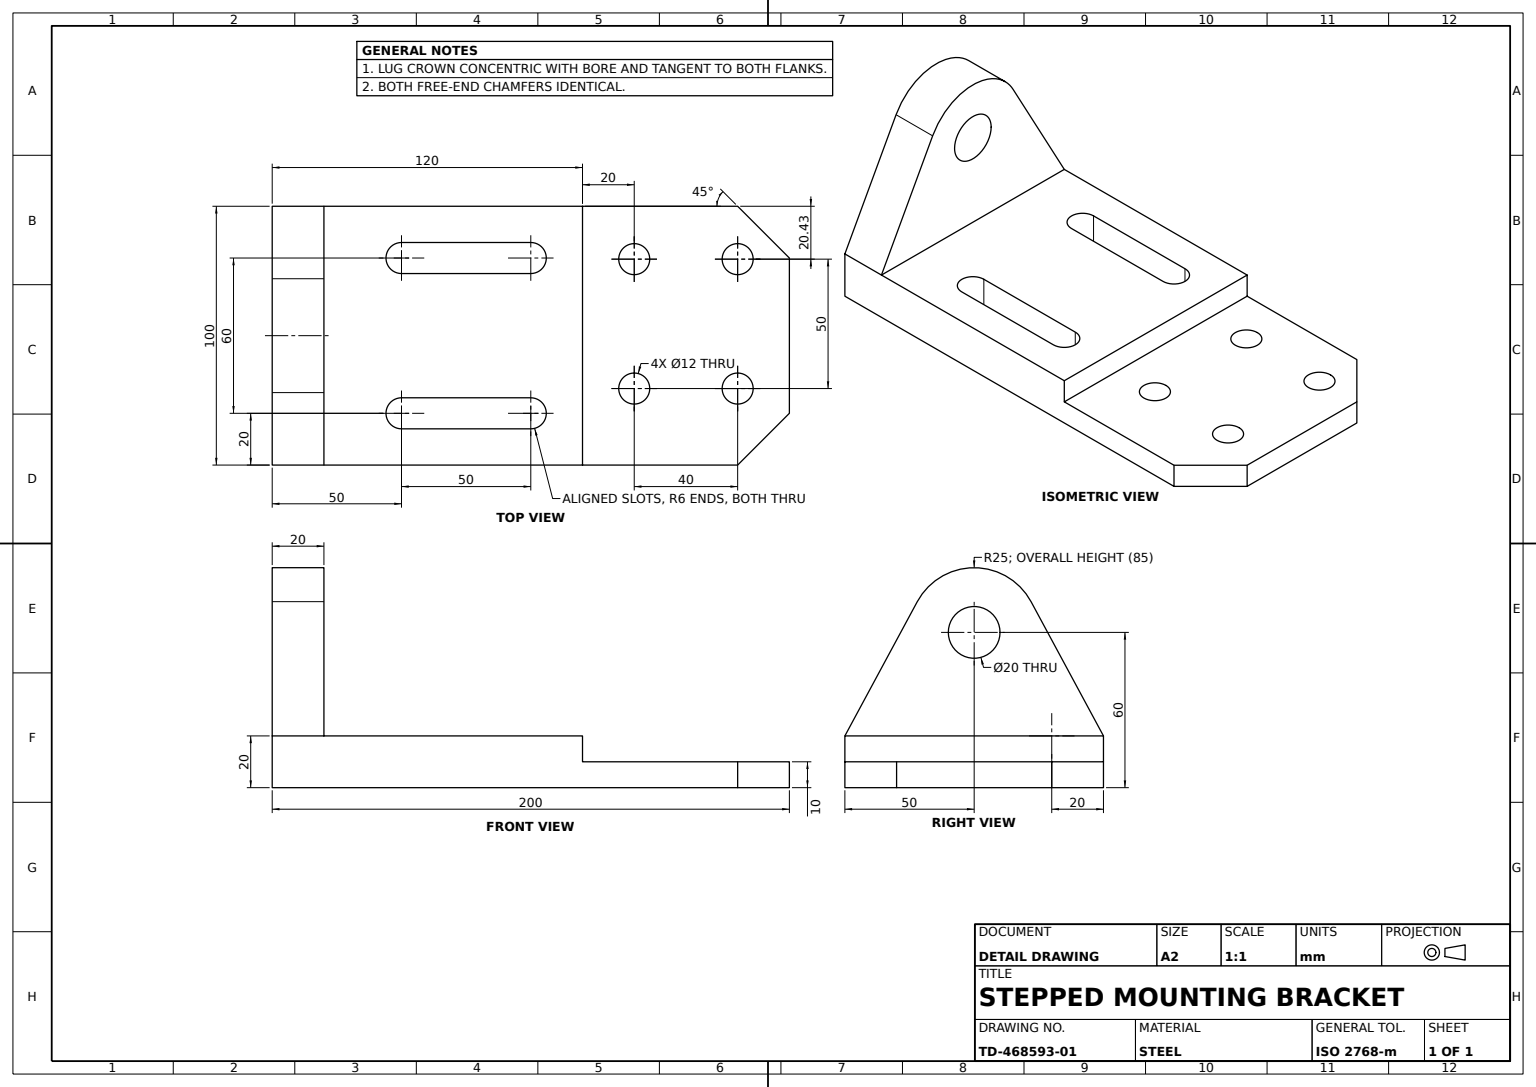
SolidWorks part; units mm, degrees
material "Plain Carbon Steel"
ref_plane "Front Plane" through (0, 0, 0) normal (0, 0, 1) x (1, 0, 0)
ref_plane "Top Plane" through (0, 0, 0) normal (0, 1, 0) x (1, 0, 0)
ref_plane "Right Plane" through (0, 0, 0) normal (1, 0, 0) x (0, 0, -1)
sketch "Base Plate Sketch" plane through (0, 0, 0) normal (0, 1, 0) x (1, 0, 0)
  line L1 (-100, -50) -> (100, -50)
  line L2 (-100, -50) -> (-100, 50)
  line L3 (-100, 50) -> (100, 50)
  line L4 (100, -50) -> (100, 50)
  line L5 (-100, -50) -> (100, 50) construction
  line L6 (-100, 50) -> (100, -50) construction
  point P0 (0, 0)
  dimension "D1" = 100
  dimension "D2" = 200
extrude "Base Plate" add sketch "Base Plate Sketch" along normal blind 10
sketch "Raised Pad Sketch" plane through (0, 10, 0) normal (0, 1, 0) x (1, 0, 0)
  line L0 (-100, -50) -> (100, -50) construction
  line L1 (-100, 50) -> (20, 50)
  line L2 (-100, 50) -> (-100, -50)
  line L3 (-100, -50) -> (20, -50)
  line L4 (20, 50) -> (20, -50)
  dimension "D1" = 120
extrude "Raised Pad" add sketch "Raised Pad Sketch" along normal blind 10
chamfer "Corner Chamfer A" distance 20 angle 45 1 edges at (100, 5, 50)
chamfer "Corner Chamfer B" distance 20 angle 45 1 edges at (100, 5, -50)
sketch "Adjustment Slots Sketch" plane through (0, 20, 0) normal (0, 1, 0) x (1, 0, 0)
  line L0 (-50, -30) -> (0, -30) construction
  line L1 (-100, -50) -> (20, -50) construction
  line L2 (-50, -24) -> (0, -24)
  line L3 (-50, -36) -> (0, -36)
  line L4 (-100, 0) -> (20, 0) construction
  line L5 (-100, 50) -> (-100, -50) construction
  line L6 (20, -50) -> (20, 50) construction
  line L7 (-50, 30) -> (0, 30) construction
  line L8 (-50, 24) -> (0, 24)
  line L9 (-50, 36) -> (0, 36)
  arc A0 (-50, -24) -> (-50, -36) centre (-50, -30) ccw
  arc A1 (0, -36) -> (0, -24) centre (0, -30) ccw
  arc A2 (-50, 24) -> (-50, 36) centre (-50, 30) cw
  arc A3 (0, 36) -> (0, 24) centre (0, 30) cw
  point P4 (-25, -30)
  point P18 (-25, 30)
  dimension "D3" = 6
  dimension "D4" = 50
  dimension "D1" = 50
  dimension "D2" = 20
extrude "Adjustment Slots 2x" cut sketch "Adjustment Slots Sketch" against normal blind 20
sketch "Lug Sketch" plane through (-100, 0, 0) normal (-1, 0, 0) x (0, 0, 1)
  line L0 (-21.9998, 71.8747) -> (-50, 20)
  line L1 (21.9998, 71.8747) -> (50, 20)
  line L2 (-50, 20) -> (50, 20)
  arc A0 (21.9998, 71.8747) -> (-21.9998, 71.8747) centre (0, 60) ccw
  circle A1 centre (0, 60) radius 10
  dimension "D1" = 50
  dimension "D2" = 20
  dimension "D3" = 60
  dimension "D4" = 50
extrude "Pierced Lug" add sketch "Lug Sketch" against normal blind 20
sketch "Mounting Holes Sketch" plane through (0, 10, 0) normal (0, 1, 0) x (1, 0, 0)
  line L1 (100, -30) -> (100, 30) construction
  line L3 (80, 50) -> (20, 50) construction
  circle A0 centre (40, 29.5656) radius 6
  circle A1 centre (80, 29.5656) radius 6
  circle A2 centre (80, -20.4344) radius 6
  circle A3 centre (40, -20.4344) radius 6
  dimension "D4" = 12
  dimension "D5" = 12
  dimension "D1" = 40
  dimension "D2" = 50
  dimension "D3" = 20
  dimension "D6" = 20.4344
extrude "Mounting Holes 4x" cut sketch "Mounting Holes Sketch" against normal blind 20
